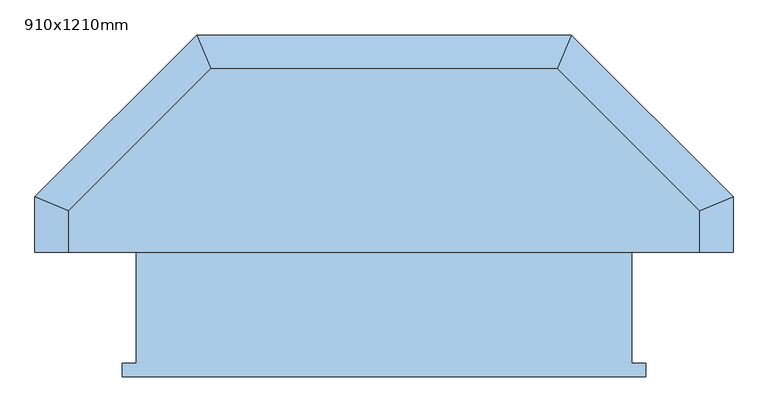
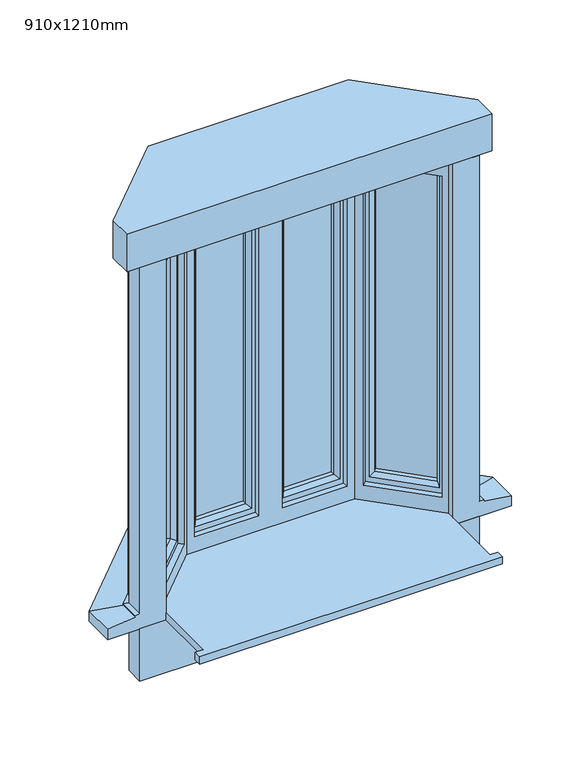
"""IFC4 building model written with IfcOpenShell, lengths in millimetres: window geometry, 910x1210mm."""

from ifc_helpers import new_model, si_unit, frame, origin, place, context, project, spatial, polyline, outline, extrude, faceted_brep, source, transform, mapped, element, save


def window_910x1210mm_154f9356(model_context):
    return source(origin(), model_context, "Body", "SolidModel", [
        extrude(outline(polyline([(-1148.0, 186.004836), (-887.4810921, 446.5237439), (-252.5189079, 446.5237439), (8.0, 186.004836), (8.0, 110.0565678), (-1148.0, 110.0565678), (-1148.0, 186.004836)])), frame((0.0, 0.0, 2110.0), z_axis=(0.0, 0.0, 1.0), x_axis=(1.0, 0.0, 0.0)), (0.0, 0.0, 1.0), 125.0),
        extrude(outline(polyline([(-32.0, 169.4362935), (-32.0, 110.0565678), (-1108.0, 110.0565678), (-1108.0, 169.4362935), (-870.9125497, 406.5237439), (-269.0874503, 406.5237439), (-32.0, 169.4362935)])), frame((0.0, 0.0, 725.0), z_axis=(0.0, 0.0, 1.0), x_axis=(1.0, 0.0, 0.0)), (0.0, 0.0, 1.0), 175.0),
        extrude(outline(polyline([(-90.0, -118.1434322), (-1050.0, -118.1434322), (-1050.0, -93.1434322), (-1025.0, -93.1434322), (-1025.0, 135.0565678), (-836.532824, 323.5237439), (-303.467176, 323.5237439), (-115.0, 135.0565678), (-115.0, -93.1434322), (-90.0, -93.1434322), (-90.0, -118.1434322)])), frame((0.0, 0.0, 900.0), z_axis=(0.0, 0.0, 1.0), x_axis=(1.0, 0.0, 0.0)), (0.0, 0.0, 1.0), 24.0),
        faceted_brep([(-1025.0, 110.0565678, 900.0), (-1025.0, 135.0565678, 900.0), (-1025.0, 135.0565678, 2110.0), (-1025.0, 110.0565678, 2110.0), (-1108.0, 110.0565678, 951.0), (-1123.0, 110.0565678, 949.68767), (-1123.0, 110.0565678, 944.7449676), (-1210.5, 110.0565678, 933.8088847), (-1210.5, 110.0565678, 900.0), (-1108.0, 110.0565678, 2110.0), (-1108.0, 169.4362935, 951.0), (-1108.0, 169.4362935, 2110.0), (-870.9125497, 406.5237439, 2110.0), (-870.9125497, 406.5237439, 951.0), (-1083.6898628, 193.7464307, 2070.0), (-1083.6898628, 193.7464307, 963.0), (-900.1724343, 377.2638592, 963.0), (-900.1724343, 377.2638592, 2070.0), (-1037.7279221, 147.7844899, 2070.0), (-1037.7279221, 147.7844899, 963.0), (-854.2104935, 331.3019184, 963.0), (-854.2104935, 331.3019184, 2070.0), (-1025.0, 160.5124119, 975.0), (-866.9384156, 318.5739964, 975.0), (-866.9384156, 318.5739964, 2050.0), (-1025.0, 160.5124119, 2050.0), (-1012.2720779, 147.7844899, 975.0), (-1012.2720779, 147.7844899, 2050.0), (-836.532824, 323.5237439, 900.0), (-836.532824, 323.5237439, 2110.0), (-854.2104935, 305.8460743, 2050.0), (-854.2104935, 305.8460743, 975.0), (-269.0874503, 406.5237439, 2110.0), (-269.0874503, 406.5237439, 951.0), (-310.467176, 406.5237439, 963.0), (-310.467176, 406.5237439, 2070.0), (-550.0, 406.5237439, 2070.0), (-550.0, 406.5237439, 963.0), (-829.532824, 406.5237439, 2070.0), (-829.532824, 406.5237439, 963.0), (-590.0, 406.5237439, 963.0), (-590.0, 406.5237439, 2070.0), (-829.532824, 341.5237439, 2070.0), (-829.532824, 341.5237439, 963.0), (-310.467176, 341.5237439, 963.0), (-550.0, 341.5237439, 963.0), (-550.0, 341.5237439, 2070.0), (-310.467176, 341.5237439, 2070.0), (-532.0, 341.5237439, 975.0), (-328.467176, 341.5237439, 975.0), (-328.467176, 341.5237439, 2050.0), (-532.0, 341.5237439, 2050.0), (-590.0, 341.5237439, 963.0), (-590.0, 341.5237439, 2070.0), (-811.532824, 341.5237439, 975.0), (-608.0, 341.5237439, 975.0), (-608.0, 341.5237439, 2050.0), (-811.532824, 341.5237439, 2050.0), (-811.532824, 323.5237439, 975.0), (-811.532824, 323.5237439, 2050.0), (-303.467176, 323.5237439, 900.0), (-303.467176, 323.5237439, 2110.0), (-608.0, 323.5237439, 2050.0), (-608.0, 323.5237439, 975.0), (-532.0, 323.5237439, 975.0), (-532.0, 323.5237439, 2050.0), (-328.467176, 323.5237439, 2050.0), (-328.467176, 323.5237439, 975.0), (-115.0, 135.0565678, 900.0), (-115.0, 135.0565678, 2110.0), (-285.7895065, 305.8460743, 975.0), (-285.7895065, 305.8460743, 2050.0), (-127.7279221, 147.7844899, 2050.0), (-127.7279221, 147.7844899, 975.0), (-32.0, 169.4362935, 2110.0), (-32.0, 169.4362935, 951.0), (-239.8275657, 377.2638592, 2070.0), (-239.8275657, 377.2638592, 963.0), (-56.3101372, 193.7464307, 963.0), (-56.3101372, 193.7464307, 2070.0), (-285.7895065, 331.3019184, 2070.0), (-285.7895065, 331.3019184, 963.0), (-102.2720779, 147.7844899, 963.0), (-102.2720779, 147.7844899, 2070.0), (-273.0615844, 318.5739964, 975.0), (-115.0, 160.5124119, 975.0), (-115.0, 160.5124119, 2050.0), (-273.0615844, 318.5739964, 2050.0), (-32.0, 110.0565678, 951.0), (-32.0, 110.0565678, 2110.0), (-115.0, 110.0565678, 900.0), (70.5, 110.0565678, 900.0), (70.5, 110.0565678, 933.8088847), (-17.0, 110.0565678, 944.7449676), (-17.0, 110.0565678, 949.68767), (-115.0, 110.0565678, 2110.0), (-1123.0, 175.6494969, 949.68767), (-1123.0, 175.6494969, 944.7449676), (-1210.5, 211.8931836, 933.8088847), (-1210.5, 211.8931836, 900.0), (-913.3694398, 509.0237439, 900.0), (-226.6305602, 509.0237439, 900.0), (70.5, 211.8931836, 900.0), (-877.1257531, 421.5237439, 949.68767), (-877.1257531, 421.5237439, 944.7449676), (-913.3694398, 509.0237439, 933.8088847), (-262.8742469, 421.5237439, 949.68767), (-262.8742469, 421.5237439, 944.7449676), (-226.6305602, 509.0237439, 933.8088847), (-17.0, 175.6494969, 949.68767), (-17.0, 175.6494969, 944.7449676), (70.5, 211.8931836, 933.8088847)], [[[0, 1, 2, 3]], [[4, 5, 6, 7, 8, 0, 3, 9]], [[10, 4, 9, 11]], [[10, 11, 12, 13], [14, 15, 16, 17]], [[15, 14, 18, 19]], [[20, 19, 18, 21], [22, 23, 24, 25]], [[26, 22, 25, 27]], [[2, 1, 28, 29], [26, 27, 30, 31]], [[23, 31, 30, 24]], [[17, 16, 20, 21]], [[13, 12, 32, 33], [34, 35, 36, 37], [38, 39, 40, 41]], [[39, 38, 42, 43]], [[44, 45, 46, 47], [48, 49, 50, 51]], [[52, 43, 42, 53], [54, 55, 56, 57]], [[58, 54, 57, 59]], [[29, 28, 60, 61], [58, 59, 62, 63], [64, 65, 66, 67]], [[61, 60, 68, 69], [70, 71, 72, 73]], [[49, 67, 66, 50]], [[35, 34, 44, 47]], [[33, 32, 74, 75], [76, 77, 78, 79]], [[77, 76, 80, 81]], [[82, 81, 80, 83], [84, 85, 86, 87]], [[70, 84, 87, 71]], [[85, 73, 72, 86]], [[79, 78, 82, 83]], [[88, 75, 74, 89]], [[90, 91, 92, 93, 94, 88, 89, 95]], [[69, 68, 90, 95]], [[41, 40, 52, 53]], [[37, 36, 46, 45]], [[64, 48, 51, 65]], [[55, 63, 62, 56]], [[26, 31, 23, 22]], [[49, 48, 64, 67]], [[55, 54, 58, 63]], [[70, 73, 85, 84]], [[16, 15, 19, 20]], [[34, 37, 45, 44]], [[40, 39, 43, 52]], [[78, 77, 81, 82]], [[5, 4, 10, 96]], [[6, 5, 96, 97]], [[7, 6, 97, 98]], [[8, 7, 98, 99]], [[0, 8, 99, 100, 101, 102, 91, 90, 68, 60, 28, 1]], [[96, 10, 13, 103]], [[97, 96, 103, 104]], [[98, 97, 104, 105]], [[99, 98, 105, 100]], [[103, 13, 33, 106]], [[104, 103, 106, 107]], [[105, 104, 107, 108]], [[101, 100, 105, 108]], [[106, 33, 75, 109]], [[107, 106, 109, 110]], [[108, 107, 110, 111]], [[102, 101, 108, 111]], [[109, 75, 88, 94]], [[110, 109, 94, 93]], [[111, 110, 93, 92]], [[91, 102, 111, 92]], [[9, 3, 2, 29, 61, 69, 95, 89, 74, 32, 12, 11]], [[14, 17, 21, 18]], [[47, 46, 36, 35]], [[53, 42, 38, 41]], [[76, 79, 83, 80]], [[25, 24, 30, 27]], [[57, 56, 62, 59]], [[66, 65, 51, 50]], [[87, 86, 72, 71]]]),
        faceted_brep([(-1090.7609307, 186.6753629, 2080.0), (-1094.8434136, 190.7578458, 2080.0), (-1094.8434136, 190.7578458, 953.0), (-1090.7609307, 186.6753629, 953.0), (-1037.7279221, 147.7844899, 2070.0), (-1083.6898628, 193.7464307, 2070.0), (-1083.6898628, 193.7464307, 963.0), (-1037.7279221, 147.7844899, 963.0), (-1019.6916786, 186.3167889, 2030.0), (-1016.6193971, 168.8930148, 2040.1480377), (-1016.6193971, 168.8930148, 992.8519623), (-1019.6916786, 186.3167889, 1003.0), (-1029.9497475, 196.5748578, 2030.0), (-1029.9497475, 196.5748578, 1003.0), (-1053.991378, 206.4743527, 2040.0), (-1037.0208153, 189.50379, 2040.0), (-1037.0208153, 189.50379, 993.0), (-1053.991378, 206.4743527, 993.0), (-1059.4880745, 226.1131848, 2030.0), (-1046.9203102, 213.5454205, 2030.0), (-1046.9203102, 213.5454205, 1003.0), (-1059.4880745, 226.1131848, 1003.0), (-1075.9065689, 217.8596562, 2047.4457548), (-1075.9065689, 217.8596562, 985.5542452), (-1091.3000258, 202.4661993, 2069.2153903), (-1091.3000258, 202.4661993, 963.7846097), (-897.1838494, 388.4174099, 953.0), (-893.1013665, 384.334927, 953.0), (-900.1724343, 377.2638592, 963.0), (-854.2104935, 331.3019184, 963.0), (-875.3190185, 310.1933935, 992.8519623), (-892.7427925, 313.265675, 1003.0), (-903.0008614, 323.5237439, 1003.0), (-895.9297936, 330.5948117, 993.0), (-912.9003563, 347.5653744, 993.0), (-919.9714242, 340.4943066, 1003.0), (-932.5391884, 353.0620709, 1003.0), (-924.2856598, 369.4805653, 985.5542452), (-908.8922029, 384.8740222, 963.7846097), (-897.1838494, 388.4174099, 2080.0), (-893.1013665, 384.334927, 2080.0), (-900.1724343, 377.2638592, 2070.0), (-854.2104935, 331.3019184, 2070.0), (-875.3190185, 310.1933935, 2040.1480377), (-892.7427925, 313.265675, 2030.0), (-903.0008614, 323.5237439, 2030.0), (-895.9297936, 330.5948117, 2040.0), (-912.9003563, 347.5653744, 2040.0), (-919.9714242, 340.4943066, 2030.0), (-932.5391884, 353.0620709, 2030.0), (-924.2856598, 369.4805653, 2047.4457548), (-908.8922029, 384.8740222, 2069.2153903)], [[[0, 1, 2, 3]], [[4, 5, 6, 7]], [[8, 9, 10, 11]], [[12, 8, 11, 13]], [[14, 15, 16, 17]], [[18, 19, 20, 21]], [[22, 18, 21, 23]], [[1, 24, 25, 2]], [[3, 2, 26, 27]], [[7, 6, 28, 29]], [[11, 10, 30, 31]], [[13, 11, 31, 32]], [[17, 16, 33, 34]], [[21, 20, 35, 36]], [[23, 21, 36, 37]], [[2, 25, 38, 26]], [[27, 26, 39, 40]], [[29, 28, 41, 42]], [[31, 30, 43, 44]], [[32, 31, 44, 45]], [[34, 33, 46, 47]], [[36, 35, 48, 49]], [[37, 36, 49, 50]], [[26, 38, 51, 39]], [[40, 39, 1, 0]], [[3, 27, 40, 0], [5, 41, 28, 6]], [[42, 41, 5, 4]], [[7, 29, 42, 4], [9, 43, 30, 10]], [[44, 43, 9, 8]], [[45, 44, 8, 12]], [[15, 46, 33, 16], [13, 32, 45, 12]], [[47, 46, 15, 14]], [[17, 34, 47, 14], [19, 48, 35, 20]], [[49, 48, 19, 18]], [[50, 49, 18, 22]], [[24, 51, 38, 25], [23, 37, 50, 22]], [[39, 51, 24, 1]]]),
        faceted_brep([(-839.532824, 406.5237439, 2080.0), (-839.532824, 412.2972465, 2080.0), (-839.532824, 412.2972465, 953.0), (-839.532824, 406.5237439, 953.0), (-829.532824, 341.5237439, 2070.0), (-829.532824, 406.5237439, 2070.0), (-829.532824, 406.5237439, 963.0), (-829.532824, 341.5237439, 963.0), (-789.532824, 356.0166437, 2030.0), (-799.6808617, 341.5237439, 2040.1480377), (-799.6808617, 341.5237439, 992.8519623), (-789.532824, 356.0166437, 1003.0), (-789.532824, 370.5237439, 2030.0), (-789.532824, 370.5237439, 1003.0), (-799.532824, 394.5237439, 2040.0), (-799.532824, 370.5237439, 2040.0), (-799.532824, 370.5237439, 993.0), (-799.532824, 394.5237439, 993.0), (-789.532824, 412.2972465, 2030.0), (-789.532824, 394.5237439, 2030.0), (-789.532824, 394.5237439, 1003.0), (-789.532824, 412.2972465, 1003.0), (-806.9785788, 418.0707492, 2047.4457548), (-806.9785788, 418.0707492, 985.5542452), (-828.7482143, 418.0707492, 2069.2153903), (-828.7482143, 418.0707492, 963.7846097), (-580.0, 412.2972465, 953.0), (-580.0, 406.5237439, 953.0), (-590.0, 406.5237439, 963.0), (-590.0, 341.5237439, 963.0), (-619.8519623, 341.5237439, 992.8519623), (-630.0, 356.0166437, 1003.0), (-630.0, 370.5237439, 1003.0), (-620.0, 370.5237439, 993.0), (-620.0, 394.5237439, 993.0), (-630.0, 394.5237439, 1003.0), (-630.0, 412.2972465, 1003.0), (-612.5542452, 418.0707492, 985.5542452), (-590.7846097, 418.0707492, 963.7846097), (-580.0, 412.2972465, 2080.0), (-580.0, 406.5237439, 2080.0), (-590.0, 406.5237439, 2070.0), (-590.0, 341.5237439, 2070.0), (-619.8519623, 341.5237439, 2040.1480377), (-630.0, 356.0166437, 2030.0), (-630.0, 370.5237439, 2030.0), (-620.0, 370.5237439, 2040.0), (-620.0, 394.5237439, 2040.0), (-630.0, 394.5237439, 2030.0), (-630.0, 412.2972465, 2030.0), (-612.5542452, 418.0707492, 2047.4457548), (-590.7846097, 418.0707492, 2069.2153903)], [[[0, 1, 2, 3]], [[4, 5, 6, 7]], [[8, 9, 10, 11]], [[12, 8, 11, 13]], [[14, 15, 16, 17]], [[18, 19, 20, 21]], [[22, 18, 21, 23]], [[1, 24, 25, 2]], [[3, 2, 26, 27]], [[7, 6, 28, 29]], [[11, 10, 30, 31]], [[13, 11, 31, 32]], [[17, 16, 33, 34]], [[21, 20, 35, 36]], [[23, 21, 36, 37]], [[2, 25, 38, 26]], [[27, 26, 39, 40]], [[29, 28, 41, 42]], [[31, 30, 43, 44]], [[32, 31, 44, 45]], [[34, 33, 46, 47]], [[36, 35, 48, 49]], [[37, 36, 49, 50]], [[26, 38, 51, 39]], [[40, 39, 1, 0]], [[3, 27, 40, 0], [5, 41, 28, 6]], [[42, 41, 5, 4]], [[7, 29, 42, 4], [9, 43, 30, 10]], [[44, 43, 9, 8]], [[45, 44, 8, 12]], [[15, 46, 33, 16], [13, 32, 45, 12]], [[47, 46, 15, 14]], [[17, 34, 47, 14], [19, 48, 35, 20]], [[49, 48, 19, 18]], [[50, 49, 18, 22]], [[24, 51, 38, 25], [23, 37, 50, 22]], [[39, 51, 24, 1]]]),
        faceted_brep([(-560.0, 406.5237439, 2080.0), (-560.0, 412.2972465, 2080.0), (-560.0, 412.2972465, 953.0), (-560.0, 406.5237439, 953.0), (-550.0, 341.5237439, 2070.0), (-550.0, 406.5237439, 2070.0), (-550.0, 406.5237439, 963.0), (-550.0, 341.5237439, 963.0), (-510.0, 356.0166437, 2030.0), (-520.1480377, 341.5237439, 2040.1480377), (-520.1480377, 341.5237439, 992.8519623), (-510.0, 356.0166437, 1003.0), (-510.0, 370.5237439, 2030.0), (-510.0, 370.5237439, 1003.0), (-520.0, 394.5237439, 2040.0), (-520.0, 370.5237439, 2040.0), (-520.0, 370.5237439, 993.0), (-520.0, 394.5237439, 993.0), (-510.0, 412.2972465, 2030.0), (-510.0, 394.5237439, 2030.0), (-510.0, 394.5237439, 1003.0), (-510.0, 412.2972465, 1003.0), (-527.4457548, 418.0707492, 2047.4457548), (-527.4457548, 418.0707492, 985.5542452), (-549.2153903, 418.0707492, 2069.2153903), (-549.2153903, 418.0707492, 963.7846097), (-300.467176, 412.2972465, 953.0), (-300.467176, 406.5237439, 953.0), (-310.467176, 406.5237439, 963.0), (-310.467176, 341.5237439, 963.0), (-340.3191383, 341.5237439, 992.8519623), (-350.467176, 356.0166437, 1003.0), (-350.467176, 370.5237439, 1003.0), (-340.467176, 370.5237439, 993.0), (-340.467176, 394.5237439, 993.0), (-350.467176, 394.5237439, 1003.0), (-350.467176, 412.2972465, 1003.0), (-333.0214212, 418.0707492, 985.5542452), (-311.2517857, 418.0707492, 963.7846097), (-300.467176, 412.2972465, 2080.0), (-300.467176, 406.5237439, 2080.0), (-310.467176, 406.5237439, 2070.0), (-310.467176, 341.5237439, 2070.0), (-340.3191383, 341.5237439, 2040.1480377), (-350.467176, 356.0166437, 2030.0), (-350.467176, 370.5237439, 2030.0), (-340.467176, 370.5237439, 2040.0), (-340.467176, 394.5237439, 2040.0), (-350.467176, 394.5237439, 2030.0), (-350.467176, 412.2972465, 2030.0), (-333.0214212, 418.0707492, 2047.4457548), (-311.2517857, 418.0707492, 2069.2153903)], [[[0, 1, 2, 3]], [[4, 5, 6, 7]], [[8, 9, 10, 11]], [[12, 8, 11, 13]], [[14, 15, 16, 17]], [[18, 19, 20, 21]], [[22, 18, 21, 23]], [[1, 24, 25, 2]], [[3, 2, 26, 27]], [[7, 6, 28, 29]], [[11, 10, 30, 31]], [[13, 11, 31, 32]], [[17, 16, 33, 34]], [[21, 20, 35, 36]], [[23, 21, 36, 37]], [[2, 25, 38, 26]], [[27, 26, 39, 40]], [[29, 28, 41, 42]], [[31, 30, 43, 44]], [[32, 31, 44, 45]], [[34, 33, 46, 47]], [[36, 35, 48, 49]], [[37, 36, 49, 50]], [[26, 38, 51, 39]], [[40, 39, 1, 0]], [[3, 27, 40, 0], [5, 41, 28, 6]], [[42, 41, 5, 4]], [[7, 29, 42, 4], [9, 43, 30, 10]], [[44, 43, 9, 8]], [[45, 44, 8, 12]], [[15, 46, 33, 16], [13, 32, 45, 12]], [[47, 46, 15, 14]], [[17, 34, 47, 14], [19, 48, 35, 20]], [[49, 48, 19, 18]], [[50, 49, 18, 22]], [[24, 51, 38, 25], [23, 37, 50, 22]], [[39, 51, 24, 1]]]),
        faceted_brep([(-246.8986335, 384.334927, 2080.0), (-242.8161506, 388.4174099, 2080.0), (-242.8161506, 388.4174099, 953.0), (-246.8986335, 384.334927, 953.0), (-285.7895065, 331.3019184, 2070.0), (-239.8275657, 377.2638592, 2070.0), (-239.8275657, 377.2638592, 963.0), (-285.7895065, 331.3019184, 963.0), (-247.2572075, 313.265675, 2030.0), (-264.6809815, 310.1933935, 2040.1480377), (-264.6809815, 310.1933935, 992.8519623), (-247.2572075, 313.265675, 1003.0), (-236.9991386, 323.5237439, 2030.0), (-236.9991386, 323.5237439, 1003.0), (-227.0996437, 347.5653744, 2040.0), (-244.0702064, 330.5948117, 2040.0), (-244.0702064, 330.5948117, 993.0), (-227.0996437, 347.5653744, 993.0), (-207.4608116, 353.0620709, 2030.0), (-220.0285758, 340.4943066, 2030.0), (-220.0285758, 340.4943066, 1003.0), (-207.4608116, 353.0620709, 1003.0), (-215.7143402, 369.4805653, 2047.4457548), (-215.7143402, 369.4805653, 985.5542452), (-231.1077971, 384.8740222, 2069.2153903), (-231.1077971, 384.8740222, 963.7846097), (-45.1565864, 190.7578458, 953.0), (-49.2390693, 186.6753629, 953.0), (-56.3101372, 193.7464307, 963.0), (-102.2720779, 147.7844899, 963.0), (-123.3806029, 168.8930148, 992.8519623), (-120.3083214, 186.3167889, 1003.0), (-110.0502525, 196.5748578, 1003.0), (-102.9791847, 189.50379, 993.0), (-86.008622, 206.4743527, 993.0), (-93.0796898, 213.5454205, 1003.0), (-80.5119255, 226.1131848, 1003.0), (-64.0934311, 217.8596562, 985.5542452), (-48.6999742, 202.4661993, 963.7846097), (-45.1565864, 190.7578458, 2080.0), (-49.2390693, 186.6753629, 2080.0), (-56.3101372, 193.7464307, 2070.0), (-102.2720779, 147.7844899, 2070.0), (-123.3806029, 168.8930148, 2040.1480377), (-120.3083214, 186.3167889, 2030.0), (-110.0502525, 196.5748578, 2030.0), (-102.9791847, 189.50379, 2040.0), (-86.008622, 206.4743527, 2040.0), (-93.0796898, 213.5454205, 2030.0), (-80.5119255, 226.1131848, 2030.0), (-64.0934311, 217.8596562, 2047.4457548), (-48.6999742, 202.4661993, 2069.2153903)], [[[0, 1, 2, 3]], [[4, 5, 6, 7]], [[8, 9, 10, 11]], [[12, 8, 11, 13]], [[14, 15, 16, 17]], [[18, 19, 20, 21]], [[22, 18, 21, 23]], [[1, 24, 25, 2]], [[3, 2, 26, 27]], [[7, 6, 28, 29]], [[11, 10, 30, 31]], [[13, 11, 31, 32]], [[17, 16, 33, 34]], [[21, 20, 35, 36]], [[23, 21, 36, 37]], [[2, 25, 38, 26]], [[27, 26, 39, 40]], [[29, 28, 41, 42]], [[31, 30, 43, 44]], [[32, 31, 44, 45]], [[34, 33, 46, 47]], [[36, 35, 48, 49]], [[37, 36, 49, 50]], [[26, 38, 51, 39]], [[40, 39, 1, 0]], [[3, 27, 40, 0], [5, 41, 28, 6]], [[42, 41, 5, 4]], [[7, 29, 42, 4], [9, 43, 30, 10]], [[44, 43, 9, 8]], [[45, 44, 8, 12]], [[15, 46, 33, 16], [13, 32, 45, 12]], [[47, 46, 15, 14]], [[17, 34, 47, 14], [19, 48, 35, 20]], [[49, 48, 19, 18]], [[50, 49, 18, 22]], [[24, 51, 38, 25], [23, 37, 50, 22]], [[39, 51, 24, 1]]]),
        extrude(outline(polyline([(-340.467176, 370.5237439), (-520.0, 370.5237439), (-520.0, 394.5237439), (-340.467176, 394.5237439), (-340.467176, 370.5237439)])), frame((0.0, 0.0, 985.5542452), z_axis=(0.0, 0.0, 1.0), x_axis=(1.0, 0.0, 0.0)), (0.0, 0.0, 1.0), 1061.8915096),
        extrude(outline(polyline([(-620.0, 370.5237439), (-799.532824, 370.5237439), (-799.532824, 394.5237439), (-620.0, 394.5237439), (-620.0, 370.5237439)])), frame((0.0, 0.0, 985.5542452), z_axis=(0.0, 0.0, 1.0), x_axis=(1.0, 0.0, 0.0)), (0.0, 0.0, 1.0), 1061.8915096),
        extrude(outline(polyline([(-1053.991378, 206.4743527), (-912.9003563, 347.5653744), (-895.9297936, 330.5948117), (-1037.0208153, 189.50379), (-1053.991378, 206.4743527)])), frame((0.0, 0.0, 992.8519623), z_axis=(0.0, 0.0, 1.0), x_axis=(1.0, 0.0, 0.0)), (0.0, 0.0, 1.0), 1047.2960754),
        extrude(outline(polyline([(-102.9791847, 189.50379), (-244.0702064, 330.5948117), (-227.0996437, 347.5653744), (-86.008622, 206.4743527), (-102.9791847, 189.50379)])), frame((0.0, 0.0, 993.0), z_axis=(0.0, 0.0, 1.0), x_axis=(1.0, 0.0, 0.0)), (0.0, 0.0, 1.0), 1047.0),
    ])


if __name__ == "__main__":
    model = new_model("IFC4")
    model_context = context("Model", 3, world=origin())
    ifc_project = project(units=[si_unit("LENGTHUNIT", "METRE", prefix="MILLI")], contexts=[model_context])
    site = spatial("IfcSite", under=ifc_project)
    building = spatial("IfcBuilding", under=site)
    placement = place(None, origin())
    window_910x1210mm_shape = window_910x1210mm_154f9356(model_context)
    element("IfcWindow", 1, ObjectType="910x1210mm", at=placement, inside=building, context=model_context, shape_type="MappedRepresentation", body=[
        mapped(window_910x1210mm_shape, transform((0.0, 0.0, 0.0), x_axis=(1.0, 0.0, 0.0), y_axis=(0.0, 1.0, 0.0), z_axis=(0.0, 0.0, 1.0))),
    ])
    save(model, "model.ifc")

# Revit data of these elements
# Type "910x1210mm"
#   Type Mark = "19"
#   Operation = "UserDefined"
#   Construction Type Id = "GSP4R"
#   Keynote = "L10"
#   Analytic Construction = "1/8 in Pilkington single glazing"
#   Wrap Layers (Ext) from Ext = 0' - 4.03543"
#   Wrap Layers (Int) from Ext = 0' - 6.98819"
#   Window Board Projection = 0' - 0.98425"
#   Window Board Extention = 0' - 0.98425"
#   Visual Light Transmittance = 0.9
#   Solar Heat Gain Coefficient = 0.78
#   Heat Transfer Coefficient (U) = 0.6496 BTU/(h·ft²·°F)
#   Glazing Thickness = 0' - 0.94488"
#   DONT CHANGE - Splay Width = 0' - 7.41997"
#   Rough Width = 2' - 11.82677"
#   Rough Height = 3' - 11.6378"
#   Roof Thickness = 0' - 4.92126"
#   Roof Overhang = 0' - 1.5748"
#   Plinth Thickness = 0' - 6.88976"
#   Height = 3' - 11.6378"
#   Width = 2' - 11.82677"
#   Frame Depth = 0' - 2.55906"
#   Default Head Height = 6' - 11.07087"
#   Cill Depth = 0' - 3.44488"
#   Cavity Closer Width = 0' - 1.9685"
#   Cavity Closer Offset from Ext = 0' - 4.03543"
#   Cavity Closer Depth = 0' - 3.34646"
#   Vis - Cavity Closers = yes
#   Define Thermal Properties by = 1
#   Material Trim = Window Frame
#   Material Glass = Glass
#   Material Frame = Window Frame
#   Manufacturer = ""
#   Wall Closure = (empty or 0)
# Element 1 (IfcWindow, "910x1210mm")
#   Materials on its faces: "Window Frame", "Glass"
# Materials
#   "Window Frame": colour RGB 249 249 249, transparency 0
#   "Glass": class "Glass", colour RGB 0 128 192, transparency 0.75, Description = "Soda Lime Glass", Cost = 0
